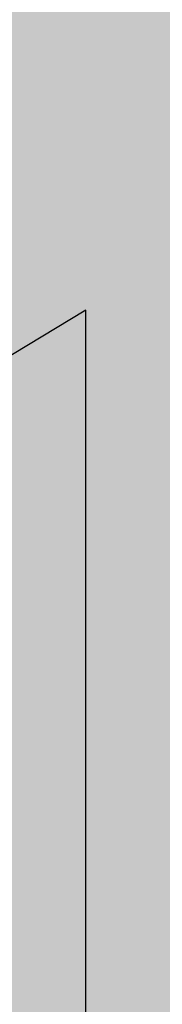
# Model space of a CAD drawing. Units: millimetres. Extents: x -22994 to 29398, y -19990 to 20176.
# Tile 79 of 135: x 225.272 to 225.543, y 85.199 to 87.071. Entities that reach past the tile are written whole.
import ezdxf
from ezdxf import colors
from ezdxf.entities.mleader import LeaderData, LeaderLine
from ezdxf.math import Vec2, Vec3

# ---------------------------------------------------------------- set-up
doc = ezdxf.new("R2010")
doc.units = ezdxf.units.MM
doc.header["$MEASUREMENT"] = 0
for name, color, linetype, lineweight in [('M-ANNO-TEXT', 7, 'Continuous', 25), ('M-DIMS', 2, 'Continuous', 18), ('M-EQPM', 7, 'Continuous', 25), ('M-EQPM-PATT', 7, 'Continuous', 18)]:
    doc.layers.add(name, color=color, linetype=linetype, lineweight=lineweight)
doc.styles.get("Standard").update_dxf_attribs({"font": 'arial.ttf'})
doc.dimstyles.get("Standard").update_dxf_attribs({"dimtxt": 0.18, "dimasz": 10000, "dimexe": 0.18, "dimexo": 0.0625, "dimgap": 0.09, "dimtad": 0, "dimtih": 1, "dimtoh": 1, "dimdec": 0, "dimzin": 0, "dimdsep": 46, "dimtxsty": 'Standard', "dimcen": 0.09, "dimadec": 0, "dimazin": 0, "dimtfac": 1, "dimtdec": 0, "dimtofl": 0, "dimtmove": 0, "dimatfit": 3, "dimfxl": 1, "dimtolj": 1, "dimtzin": 0, "dimlwd": 30, "dimarcsym": 0})

# ---------------------------------------------------------------- blocks, each defined once
blk = doc.blocks.new('*D2')
at = {"layer": 'Defpoints', "color": 0, "transparency": 16777216}
for p in [(6.6773, 10.2713), (290.852, 10.2713), (290.852, -5.0787)]:
    blk.add_point(p, dxfattribs=at)
at = {"layer": 'M-DIMS', "color": 0, "lineweight": -2, "transparency": 16777216}
for p, q in [((6.6773, 10.2088), (6.6773, -5.2587)), ((290.852, 10.2088), (290.852, -5.2587))]:
    blk.add_line(p, q, dxfattribs=at)
at = {"layer": 'M-DIMS', "color": 0, "lineweight": 30, "transparency": 16777216}
for p, q in [((-9993.3227, -5.0787), (-19993.3227, -5.0787)), ((10290.852, -5.0787), (20290.852, -5.0787))]:
    blk.add_line(p, q, dxfattribs=at)
at = {"layer": 'M-DIMS', "color": 0, "transparency": 16777216}
for points in [[(-9993.3227, 1661.5879), (-9993.3227, -1671.7454), (6.6773, -5.0787)], [(10290.852, 1661.5879), (10290.852, -1671.7454), (290.852, -5.0787)]]:
    blk.add_solid(points, dxfattribs=at)
at = {"layer": 'M-DIMS', "color": 0, "transparency": 16777216, "insert": (148.7647, -5.0787), "char_height": 0.18, "attachment_point": 5}
blk.add_mtext('\\A1;284.2', dxfattribs=at)
blk = doc.blocks.new('*D3')
at = {"layer": 'Defpoints', "color": 0, "transparency": 16777216}
for p in [(110.2647, 204.1654), (110.2647, 176.3662), (95.8327, 127.967)]:
    blk.add_point(p, dxfattribs=at)
at = {"layer": 'M-DIMS', "color": 0, "lineweight": -2, "transparency": 16777216}
for p, q in [((95.8327, 128.0295), (95.8327, 204.3454)), ((110.2647, 176.4287), (110.2647, 204.3454))]:
    blk.add_line(p, q, dxfattribs=at)
at = {"layer": 'M-DIMS', "color": 0, "lineweight": 30, "transparency": 16777216}
for p, q in [((-9904.1673, 204.1654), (-19904.1673, 204.1654)), ((10110.2647, 204.1654), (20110.2647, 204.1654))]:
    blk.add_line(p, q, dxfattribs=at)
at = {"layer": 'M-DIMS', "color": 0, "transparency": 16777216}
for points in [[(-9904.1673, 1870.8321), (-9904.1673, -1462.5013), (95.8327, 204.1654)], [(10110.2647, 1870.8321), (10110.2647, -1462.5013), (110.2647, 204.1654)]]:
    blk.add_solid(points, dxfattribs=at)
at = {"layer": 'M-DIMS', "color": 0, "transparency": 16777216, "insert": (103.0487, 204.1654), "char_height": 0.18, "attachment_point": 5}
blk.add_mtext('\\A1;14.432', dxfattribs=at)
blk = doc.blocks.new('*D4')
at = {"layer": 'Defpoints', "color": 0, "transparency": 16777216}
for p in [(116.2647, 204.1654), (110.2647, 176.3662), (116.2647, 176.3662)]:
    blk.add_point(p, dxfattribs=at)
at = {"layer": 'M-DIMS', "color": 0, "lineweight": -2, "transparency": 16777216}
for p, q in [((110.2647, 176.4287), (110.2647, 204.3454)), ((116.2647, 176.4287), (116.2647, 204.3454))]:
    blk.add_line(p, q, dxfattribs=at)
at = {"layer": 'M-DIMS', "color": 0, "lineweight": 30, "transparency": 16777216}
for p, q in [((-9889.7353, 204.1654), (-19889.7353, 204.1654)), ((10116.2647, 204.1654), (20116.2647, 204.1654))]:
    blk.add_line(p, q, dxfattribs=at)
at = {"layer": 'M-DIMS', "color": 0, "transparency": 16777216}
for points in [[(-9889.7353, 1870.8321), (-9889.7353, -1462.5013), (110.2647, 204.1654)], [(10116.2647, 1870.8321), (10116.2647, -1462.5013), (116.2647, 204.1654)]]:
    blk.add_solid(points, dxfattribs=at)
at = {"layer": 'M-DIMS', "color": 0, "transparency": 16777216, "insert": (113.2647, 204.1654), "char_height": 0.18, "attachment_point": 5}
blk.add_mtext('\\A1;6', dxfattribs=at)
blk = doc.blocks.new('*D5')
at = {"layer": 'Defpoints', "color": 0, "transparency": 16777216}
for p in [(181.2647, 204.1654), (116.2647, 176.3662), (181.2647, 176.3662)]:
    blk.add_point(p, dxfattribs=at)
at = {"layer": 'M-DIMS', "color": 0, "lineweight": -2, "transparency": 16777216}
for p, q in [((116.2647, 176.4287), (116.2647, 204.3454)), ((181.2647, 176.4287), (181.2647, 204.3454))]:
    blk.add_line(p, q, dxfattribs=at)
at = {"layer": 'M-DIMS', "color": 0, "lineweight": 30, "transparency": 16777216}
for p, q in [((-9883.7353, 204.1654), (-19883.7353, 204.1654)), ((10181.2647, 204.1654), (20181.2647, 204.1654))]:
    blk.add_line(p, q, dxfattribs=at)
at = {"layer": 'M-DIMS', "color": 0, "transparency": 16777216}
for points in [[(-9883.7353, 1870.8321), (-9883.7353, -1462.5013), (116.2647, 204.1654)], [(10181.2647, 1870.8321), (10181.2647, -1462.5013), (181.2647, 204.1654)]]:
    blk.add_solid(points, dxfattribs=at)
at = {"layer": 'M-DIMS', "color": 0, "transparency": 16777216, "insert": (148.7647, 204.1654), "char_height": 0.18, "attachment_point": 5}
blk.add_mtext('\\A1;65', dxfattribs=at)
blk = doc.blocks.new('*D6')
at = {"layer": 'Defpoints', "color": 0, "transparency": 16777216}
for p in [(187.2647, 204.1654), (181.2647, 176.3662), (187.2647, 176.3662)]:
    blk.add_point(p, dxfattribs=at)
at = {"layer": 'M-DIMS', "color": 0, "lineweight": -2, "transparency": 16777216}
for p, q in [((181.2647, 176.4287), (181.2647, 204.3454)), ((187.2647, 176.4287), (187.2647, 204.3454))]:
    blk.add_line(p, q, dxfattribs=at)
at = {"layer": 'M-DIMS', "color": 0, "lineweight": 30, "transparency": 16777216}
for p, q in [((-9818.7353, 204.1654), (-19818.7353, 204.1654)), ((10187.2647, 204.1654), (20187.2647, 204.1654))]:
    blk.add_line(p, q, dxfattribs=at)
at = {"layer": 'M-DIMS', "color": 0, "transparency": 16777216}
for points in [[(-9818.7353, 1870.8321), (-9818.7353, -1462.5013), (181.2647, 204.1654)], [(10187.2647, 1870.8321), (10187.2647, -1462.5013), (187.2647, 204.1654)]]:
    blk.add_solid(points, dxfattribs=at)
at = {"layer": 'M-DIMS', "color": 0, "transparency": 16777216, "insert": (184.2647, 204.1654), "char_height": 0.18, "attachment_point": 5}
blk.add_mtext('\\A1;6', dxfattribs=at)
blk = doc.blocks.new('*D7')
at = {"layer": 'Defpoints', "color": 0, "transparency": 16777216}
for p in [(201.6967, 204.1654), (187.2647, 176.3662), (201.6967, 127.967)]:
    blk.add_point(p, dxfattribs=at)
at = {"layer": 'M-DIMS', "color": 0, "lineweight": -2, "transparency": 16777216}
for p, q in [((187.2647, 176.4287), (187.2647, 204.3454)), ((201.6967, 128.0295), (201.6967, 204.3454))]:
    blk.add_line(p, q, dxfattribs=at)
at = {"layer": 'M-DIMS', "color": 0, "lineweight": 30, "transparency": 16777216}
for p, q in [((-9812.7353, 204.1654), (-19812.7353, 204.1654)), ((10201.6967, 204.1654), (20201.6967, 204.1654))]:
    blk.add_line(p, q, dxfattribs=at)
at = {"layer": 'M-DIMS', "color": 0, "transparency": 16777216}
for points in [[(-9812.7353, 1870.8321), (-9812.7353, -1462.5013), (187.2647, 204.1654)], [(10201.6967, 1870.8321), (10201.6967, -1462.5013), (201.6967, 204.1654)]]:
    blk.add_solid(points, dxfattribs=at)
at = {"layer": 'M-DIMS', "color": 0, "transparency": 16777216, "insert": (194.4807, 204.1654), "char_height": 0.18, "attachment_point": 5}
blk.add_mtext('\\A1;14.432', dxfattribs=at)
blk = doc.blocks.new('*D8')
at = {"layer": 'Defpoints', "color": 0, "transparency": 16777216}
for p in [(227.6485, 204.1654), (227.6485, 146.7296), (201.6967, 127.967)]:
    blk.add_point(p, dxfattribs=at)
at = {"layer": 'M-DIMS', "color": 0, "lineweight": -2, "transparency": 16777216}
for p, q in [((201.6967, 128.0295), (201.6967, 204.3454)), ((227.6485, 146.7921), (227.6485, 204.3454))]:
    blk.add_line(p, q, dxfattribs=at)
at = {"layer": 'M-DIMS', "color": 0, "lineweight": 30, "transparency": 16777216}
for p, q in [((-9798.3033, 204.1654), (-19798.3033, 204.1654)), ((10227.6485, 204.1654), (20227.6485, 204.1654))]:
    blk.add_line(p, q, dxfattribs=at)
at = {"layer": 'M-DIMS', "color": 0, "transparency": 16777216}
for points in [[(-9798.3033, 1870.8321), (-9798.3033, -1462.5013), (201.6967, 204.1654)], [(10227.6485, 1870.8321), (10227.6485, -1462.5013), (227.6485, 204.1654)]]:
    blk.add_solid(points, dxfattribs=at)
at = {"layer": 'M-DIMS', "color": 0, "transparency": 16777216, "insert": (214.6726, 204.1654), "char_height": 0.18, "attachment_point": 5}
blk.add_mtext('\\A1;25.95', dxfattribs=at)
blk = doc.blocks.new('*D9')
at = {"layer": 'Defpoints', "color": 0, "transparency": 16777216}
for p in [(187.2647, 176.3662), (306.202, 176.3662), (290.852, 10.2713)]:
    blk.add_point(p, dxfattribs=at)
at = {"layer": 'M-DIMS', "color": 0, "lineweight": 30, "transparency": 16777216}
for p, q in [((306.202, 10176.3662), (306.202, 20176.3662)), ((306.202, -9989.7287), (306.202, -19989.7287))]:
    blk.add_line(p, q, dxfattribs=at)
at = {"layer": 'M-DIMS', "color": 0, "lineweight": -2, "transparency": 16777216}
for p, q in [((187.3272, 176.3662), (306.382, 176.3662)), ((290.9145, 10.2713), (306.382, 10.2713))]:
    blk.add_line(p, q, dxfattribs=at)
at = {"layer": 'M-DIMS', "color": 0, "transparency": 16777216}
for points in [[(-1360.4646, 10176.3662), (1972.8687, 10176.3662), (306.202, 176.3662)], [(-1360.4646, -9989.7287), (1972.8687, -9989.7287), (306.202, 10.2713)]]:
    blk.add_solid(points, dxfattribs=at)
at = {"layer": 'M-DIMS', "color": 0, "transparency": 16777216, "insert": (306.202, 93.3187), "char_height": 0.18, "attachment_point": 5}
blk.add_mtext('\\A1;166.1', dxfattribs=at)
blk = doc.blocks.new('*D10')
at = {"layer": 'Defpoints', "color": 0, "transparency": 16777216}
for p in [(125.6498, 136.0713), (133.3459, 136.0713), (133.3459, -5.0787)]:
    blk.add_point(p, dxfattribs=at)
at = {"layer": 'M-DIMS', "color": 0, "lineweight": -2, "transparency": 16777216}
for p, q in [((125.6498, 136.0088), (125.6498, -5.2587)), ((133.3459, 136.0088), (133.3459, -5.2587))]:
    blk.add_line(p, q, dxfattribs=at)
at = {"layer": 'M-DIMS', "color": 0, "lineweight": 30, "transparency": 16777216}
for p, q in [((-9874.3502, -5.0787), (-19874.3502, -5.0787)), ((10133.3459, -5.0787), (20133.3459, -5.0787))]:
    blk.add_line(p, q, dxfattribs=at)
at = {"layer": 'M-DIMS', "color": 0, "transparency": 16777216}
for points in [[(-9874.3502, 1661.5879), (-9874.3502, -1671.7454), (125.6498, -5.0787)], [(10133.3459, 1661.5879), (10133.3459, -1671.7454), (133.3459, -5.0787)]]:
    blk.add_solid(points, dxfattribs=at)
at = {"layer": 'M-DIMS', "color": 0, "transparency": 16777216, "insert": (129.4978, -5.0787), "char_height": 0.18, "attachment_point": 5}
blk.add_mtext('\\A1;7.696', dxfattribs=at)
blk = doc.blocks.new('*D11')
at = {"layer": 'Defpoints', "color": 0, "transparency": 16777216}
for p in [(133.3459, 136.0713), (135.6498, 136.0713), (135.6498, -5.0787)]:
    blk.add_point(p, dxfattribs=at)
at = {"layer": 'M-DIMS', "color": 0, "lineweight": -2, "transparency": 16777216}
for p, q in [((133.3459, 136.0088), (133.3459, -5.2587)), ((135.6498, 136.0088), (135.6498, -5.2587))]:
    blk.add_line(p, q, dxfattribs=at)
at = {"layer": 'M-DIMS', "color": 0, "lineweight": 30, "transparency": 16777216}
for p, q in [((-9866.6541, -5.0787), (-19866.6541, -5.0787)), ((10135.6498, -5.0787), (20135.6498, -5.0787))]:
    blk.add_line(p, q, dxfattribs=at)
at = {"layer": 'M-DIMS', "color": 0, "transparency": 16777216}
for points in [[(-9866.6541, 1661.5879), (-9866.6541, -1671.7454), (133.3459, -5.0787)], [(10135.6498, 1661.5879), (10135.6498, -1671.7454), (135.6498, -5.0787)]]:
    blk.add_solid(points, dxfattribs=at)
at = {"layer": 'M-DIMS', "color": 0, "transparency": 16777216, "insert": (134.4978, -5.0787), "char_height": 0.18, "attachment_point": 5}
blk.add_mtext('\\A1;2.304', dxfattribs=at)
blk = doc.blocks.new('*D12')
at = {"layer": 'Defpoints', "color": 0, "transparency": 16777216}
for p in [(135.6498, 136.0713), (145.6498, 136.0713), (145.6498, -5.0787)]:
    blk.add_point(p, dxfattribs=at)
at = {"layer": 'M-DIMS', "color": 0, "lineweight": -2, "transparency": 16777216}
for p, q in [((135.6498, 136.0088), (135.6498, -5.2587)), ((145.6498, 136.0088), (145.6498, -5.2587))]:
    blk.add_line(p, q, dxfattribs=at)
at = {"layer": 'M-DIMS', "color": 0, "lineweight": 30, "transparency": 16777216}
for p, q in [((-9864.3502, -5.0787), (-19864.3502, -5.0787)), ((10145.6498, -5.0787), (20145.6498, -5.0787))]:
    blk.add_line(p, q, dxfattribs=at)
at = {"layer": 'M-DIMS', "color": 0, "transparency": 16777216}
for points in [[(-9864.3502, 1661.5879), (-9864.3502, -1671.7454), (135.6498, -5.0787)], [(10145.6498, 1661.5879), (10145.6498, -1671.7454), (145.6498, -5.0787)]]:
    blk.add_solid(points, dxfattribs=at)
at = {"layer": 'M-DIMS', "color": 0, "transparency": 16777216, "insert": (140.6498, -5.0787), "char_height": 0.18, "attachment_point": 5}
blk.add_mtext('\\A1;10', dxfattribs=at)
blk = doc.blocks.new('*D13')
at = {"layer": 'Defpoints', "color": 0, "transparency": 16777216}
for p in [(145.6498, 136.0713), (155.6498, 136.0713), (155.6498, -5.0787)]:
    blk.add_point(p, dxfattribs=at)
at = {"layer": 'M-DIMS', "color": 0, "lineweight": -2, "transparency": 16777216}
for p, q in [((145.6498, 136.0088), (145.6498, -5.2587)), ((155.6498, 136.0088), (155.6498, -5.2587))]:
    blk.add_line(p, q, dxfattribs=at)
at = {"layer": 'M-DIMS', "color": 0, "lineweight": 30, "transparency": 16777216}
for p, q in [((-9854.3502, -5.0787), (-19854.3502, -5.0787)), ((10155.6498, -5.0787), (20155.6498, -5.0787))]:
    blk.add_line(p, q, dxfattribs=at)
at = {"layer": 'M-DIMS', "color": 0, "transparency": 16777216}
for points in [[(-9854.3502, 1661.5879), (-9854.3502, -1671.7454), (145.6498, -5.0787)], [(10155.6498, 1661.5879), (10155.6498, -1671.7454), (155.6498, -5.0787)]]:
    blk.add_solid(points, dxfattribs=at)
at = {"layer": 'M-DIMS', "color": 0, "transparency": 16777216, "insert": (150.6498, -5.0787), "char_height": 0.18, "attachment_point": 5}
blk.add_mtext('\\A1;10', dxfattribs=at)
blk = doc.blocks.new('*D14')
at = {"layer": 'Defpoints', "color": 0, "transparency": 16777216}
for p in [(155.6498, 136.0713), (165.6498, 136.0713), (165.6498, -5.0787)]:
    blk.add_point(p, dxfattribs=at)
at = {"layer": 'M-DIMS', "color": 0, "lineweight": -2, "transparency": 16777216}
for p, q in [((155.6498, 136.0088), (155.6498, -5.2587)), ((165.6498, 136.0088), (165.6498, -5.2587))]:
    blk.add_line(p, q, dxfattribs=at)
at = {"layer": 'M-DIMS', "color": 0, "lineweight": 30, "transparency": 16777216}
for p, q in [((-9844.3502, -5.0787), (-19844.3502, -5.0787)), ((10165.6498, -5.0787), (20165.6498, -5.0787))]:
    blk.add_line(p, q, dxfattribs=at)
at = {"layer": 'M-DIMS', "color": 0, "transparency": 16777216}
for points in [[(-9844.3502, 1661.5879), (-9844.3502, -1671.7454), (155.6498, -5.0787)], [(10165.6498, 1661.5879), (10165.6498, -1671.7454), (165.6498, -5.0787)]]:
    blk.add_solid(points, dxfattribs=at)
at = {"layer": 'M-DIMS', "color": 0, "transparency": 16777216, "insert": (160.6498, -5.0787), "char_height": 0.18, "attachment_point": 5}
blk.add_mtext('\\A1;10', dxfattribs=at)
blk = doc.blocks.new('*D15')
at = {"layer": 'Defpoints', "color": 0, "transparency": 16777216}
for p in [(173.3459, 154.788), (173.3459, 136.0713), (306.202, 136.0713)]:
    blk.add_point(p, dxfattribs=at)
at = {"layer": 'M-DIMS', "color": 0, "lineweight": 30, "transparency": 16777216}
for p, q in [((306.202, 10154.788), (306.202, 20154.788)), ((306.202, -9863.9287), (306.202, -19863.9287))]:
    blk.add_line(p, q, dxfattribs=at)
at = {"layer": 'M-DIMS', "color": 0, "lineweight": -2, "transparency": 16777216}
for p, q in [((173.4084, 154.788), (306.382, 154.788)), ((173.4084, 136.0713), (306.382, 136.0713))]:
    blk.add_line(p, q, dxfattribs=at)
at = {"layer": 'M-DIMS', "color": 0, "transparency": 16777216}
for points in [[(-1360.4646, 10154.788), (1972.8687, 10154.788), (306.202, 154.788)], [(-1360.4646, -9863.9287), (1972.8687, -9863.9287), (306.202, 136.0713)]]:
    blk.add_solid(points, dxfattribs=at)
at = {"layer": 'M-DIMS', "color": 0, "transparency": 16777216, "insert": (306.202, 145.4297), "char_height": 0.18, "attachment_point": 5}
blk.add_mtext('\\A1;18.717', dxfattribs=at)
blk = doc.blocks.new('*D16')
at = {"layer": 'Defpoints', "color": 0, "transparency": 16777216}
for p in [(120.1702, 204.1654), (110.4658, 48.0349), (120.1702, 48.0349)]:
    blk.add_point(p, dxfattribs=at)
at = {"layer": 'M-DIMS', "color": 0, "lineweight": -2, "transparency": 16777216}
for p, q in [((110.4658, 48.0974), (110.4658, 204.3454)), ((120.1702, 48.0974), (120.1702, 204.3454))]:
    blk.add_line(p, q, dxfattribs=at)
at = {"layer": 'M-DIMS', "color": 0, "lineweight": 30, "transparency": 16777216}
for p, q in [((-9889.5342, 204.1654), (-19889.5342, 204.1654)), ((10120.1702, 204.1654), (20120.1702, 204.1654))]:
    blk.add_line(p, q, dxfattribs=at)
at = {"layer": 'M-DIMS', "color": 0, "transparency": 16777216}
for points in [[(-9889.5342, 1870.8321), (-9889.5342, -1462.5013), (110.4658, 204.1654)], [(10120.1702, 1870.8321), (10120.1702, -1462.5013), (120.1702, 204.1654)]]:
    blk.add_solid(points, dxfattribs=at)
at = {"layer": 'M-DIMS', "color": 0, "transparency": 16777216, "insert": (115.318, 204.1654), "char_height": 0.18, "attachment_point": 5}
blk.add_mtext('\\A1;9.704', dxfattribs=at)
blk = doc.blocks.new('*D17')
at = {"layer": 'Defpoints', "color": 0, "transparency": 16777216}
for p in [(126.1702, 204.1654), (120.1702, 48.0349), (126.1702, 48.0349)]:
    blk.add_point(p, dxfattribs=at)
at = {"layer": 'M-DIMS', "color": 0, "lineweight": -2, "transparency": 16777216}
for p, q in [((120.1702, 48.0974), (120.1702, 204.3454)), ((126.1702, 48.0974), (126.1702, 204.3454))]:
    blk.add_line(p, q, dxfattribs=at)
at = {"layer": 'M-DIMS', "color": 0, "lineweight": 30, "transparency": 16777216}
for p, q in [((-9879.8298, 204.1654), (-19879.8298, 204.1654)), ((10126.1702, 204.1654), (20126.1702, 204.1654))]:
    blk.add_line(p, q, dxfattribs=at)
at = {"layer": 'M-DIMS', "color": 0, "transparency": 16777216}
for points in [[(-9879.8298, 1870.8321), (-9879.8298, -1462.5013), (120.1702, 204.1654)], [(10126.1702, 1870.8321), (10126.1702, -1462.5013), (126.1702, 204.1654)]]:
    blk.add_solid(points, dxfattribs=at)
at = {"layer": 'M-DIMS', "color": 0, "transparency": 16777216, "insert": (123.1702, 204.1654), "char_height": 0.18, "attachment_point": 5}
blk.add_mtext('\\A1;6', dxfattribs=at)
blk = doc.blocks.new('*D18')
at = {"layer": 'Defpoints', "color": 0, "transparency": 16777216}
for p in [(132.1702, 204.1654), (126.1702, 48.0349), (132.1702, 48.0349)]:
    blk.add_point(p, dxfattribs=at)
at = {"layer": 'M-DIMS', "color": 0, "lineweight": -2, "transparency": 16777216}
for p, q in [((126.1702, 48.0974), (126.1702, 204.3454)), ((132.1702, 48.0974), (132.1702, 204.3454))]:
    blk.add_line(p, q, dxfattribs=at)
at = {"layer": 'M-DIMS', "color": 0, "lineweight": 30, "transparency": 16777216}
for p, q in [((-9873.8298, 204.1654), (-19873.8298, 204.1654)), ((10132.1702, 204.1654), (20132.1702, 204.1654))]:
    blk.add_line(p, q, dxfattribs=at)
at = {"layer": 'M-DIMS', "color": 0, "transparency": 16777216}
for points in [[(-9873.8298, 1870.8321), (-9873.8298, -1462.5013), (126.1702, 204.1654)], [(10132.1702, 1870.8321), (10132.1702, -1462.5013), (132.1702, 204.1654)]]:
    blk.add_solid(points, dxfattribs=at)
at = {"layer": 'M-DIMS', "color": 0, "transparency": 16777216, "insert": (129.1702, 204.1654), "char_height": 0.18, "attachment_point": 5}
blk.add_mtext('\\A1;6', dxfattribs=at)
blk = doc.blocks.new('*D19')
at = {"layer": 'Defpoints', "color": 0, "transparency": 16777216}
for p in [(138.1702, 204.1654), (132.1702, 48.0349), (138.1702, 48.0349)]:
    blk.add_point(p, dxfattribs=at)
at = {"layer": 'M-DIMS', "color": 0, "lineweight": -2, "transparency": 16777216}
for p, q in [((132.1702, 48.0974), (132.1702, 204.3454)), ((138.1702, 48.0974), (138.1702, 204.3454))]:
    blk.add_line(p, q, dxfattribs=at)
at = {"layer": 'M-DIMS', "color": 0, "lineweight": 30, "transparency": 16777216}
for p, q in [((-9867.8298, 204.1654), (-19867.8298, 204.1654)), ((10138.1702, 204.1654), (20138.1702, 204.1654))]:
    blk.add_line(p, q, dxfattribs=at)
at = {"layer": 'M-DIMS', "color": 0, "transparency": 16777216}
for points in [[(-9867.8298, 1870.8321), (-9867.8298, -1462.5013), (132.1702, 204.1654)], [(10138.1702, 1870.8321), (10138.1702, -1462.5013), (138.1702, 204.1654)]]:
    blk.add_solid(points, dxfattribs=at)
at = {"layer": 'M-DIMS', "color": 0, "transparency": 16777216, "insert": (135.1702, 204.1654), "char_height": 0.18, "attachment_point": 5}
blk.add_mtext('\\A1;6', dxfattribs=at)
blk = doc.blocks.new('*D20')
at = {"layer": 'Defpoints', "color": 0, "transparency": 16777216}
for p in [(144.1702, 204.1654), (138.1702, 48.0349), (144.1702, 48.0349)]:
    blk.add_point(p, dxfattribs=at)
at = {"layer": 'M-DIMS', "color": 0, "lineweight": -2, "transparency": 16777216}
for p, q in [((138.1702, 48.0974), (138.1702, 204.3454)), ((144.1702, 48.0974), (144.1702, 204.3454))]:
    blk.add_line(p, q, dxfattribs=at)
at = {"layer": 'M-DIMS', "color": 0, "lineweight": 30, "transparency": 16777216}
for p, q in [((-9861.8298, 204.1654), (-19861.8298, 204.1654)), ((10144.1702, 204.1654), (20144.1702, 204.1654))]:
    blk.add_line(p, q, dxfattribs=at)
at = {"layer": 'M-DIMS', "color": 0, "transparency": 16777216}
for points in [[(-9861.8298, 1870.8321), (-9861.8298, -1462.5013), (138.1702, 204.1654)], [(10144.1702, 1870.8321), (10144.1702, -1462.5013), (144.1702, 204.1654)]]:
    blk.add_solid(points, dxfattribs=at)
at = {"layer": 'M-DIMS', "color": 0, "transparency": 16777216, "insert": (141.1702, 204.1654), "char_height": 0.18, "attachment_point": 5}
blk.add_mtext('\\A1;6', dxfattribs=at)
blk = doc.blocks.new('*D21')
at = {"layer": 'Defpoints', "color": 0, "transparency": 16777216}
for p in [(149.1157, 204.1654), (144.1702, 48.0349), (149.1157, 48.0349)]:
    blk.add_point(p, dxfattribs=at)
at = {"layer": 'M-DIMS', "color": 0, "lineweight": -2, "transparency": 16777216}
for p, q in [((144.1702, 48.0974), (144.1702, 204.3454)), ((149.1157, 48.0974), (149.1157, 204.3454))]:
    blk.add_line(p, q, dxfattribs=at)
at = {"layer": 'M-DIMS', "color": 0, "lineweight": 30, "transparency": 16777216}
for p, q in [((-9855.8298, 204.1654), (-19855.8298, 204.1654)), ((10149.1157, 204.1654), (20149.1157, 204.1654))]:
    blk.add_line(p, q, dxfattribs=at)
at = {"layer": 'M-DIMS', "color": 0, "transparency": 16777216}
for points in [[(-9855.8298, 1870.8321), (-9855.8298, -1462.5013), (144.1702, 204.1654)], [(10149.1157, 1870.8321), (10149.1157, -1462.5013), (149.1157, 204.1654)]]:
    blk.add_solid(points, dxfattribs=at)
at = {"layer": 'M-DIMS', "color": 0, "transparency": 16777216, "insert": (146.6429, 204.1654), "char_height": 0.18, "attachment_point": 5}
blk.add_mtext('\\A1;4.945', dxfattribs=at)
blk = doc.blocks.new('*D22')
at = {"layer": 'Defpoints', "color": 0, "transparency": 16777216}
for p in [(149.1157, 30.9895), (155.1157, 30.9895), (155.1157, -5.0787)]:
    blk.add_point(p, dxfattribs=at)
at = {"layer": 'M-DIMS', "color": 0, "lineweight": -2, "transparency": 16777216}
for p, q in [((149.1157, 30.927), (149.1157, -5.2587)), ((155.1157, 30.927), (155.1157, -5.2587))]:
    blk.add_line(p, q, dxfattribs=at)
at = {"layer": 'M-DIMS', "color": 0, "lineweight": 30, "transparency": 16777216}
for p, q in [((-9850.8843, -5.0787), (-19850.8843, -5.0787)), ((10155.1157, -5.0787), (20155.1157, -5.0787))]:
    blk.add_line(p, q, dxfattribs=at)
at = {"layer": 'M-DIMS', "color": 0, "transparency": 16777216}
for points in [[(-9850.8843, 1661.5879), (-9850.8843, -1671.7454), (149.1157, -5.0787)], [(10155.1157, 1661.5879), (10155.1157, -1671.7454), (155.1157, -5.0787)]]:
    blk.add_solid(points, dxfattribs=at)
at = {"layer": 'M-DIMS', "color": 0, "transparency": 16777216, "insert": (152.1157, -5.0787), "char_height": 0.18, "attachment_point": 5}
blk.add_mtext('\\A1;6', dxfattribs=at)
blk = doc.blocks.new('*D23')
at = {"layer": 'Defpoints', "color": 0, "transparency": 16777216}
for p in [(155.1157, 30.9895), (161.1157, 30.9895), (161.1157, -5.0787)]:
    blk.add_point(p, dxfattribs=at)
at = {"layer": 'M-DIMS', "color": 0, "lineweight": -2, "transparency": 16777216}
for p, q in [((155.1157, 30.927), (155.1157, -5.2587)), ((161.1157, 30.927), (161.1157, -5.2587))]:
    blk.add_line(p, q, dxfattribs=at)
at = {"layer": 'M-DIMS', "color": 0, "lineweight": 30, "transparency": 16777216}
for p, q in [((-9844.8843, -5.0787), (-19844.8843, -5.0787)), ((10161.1157, -5.0787), (20161.1157, -5.0787))]:
    blk.add_line(p, q, dxfattribs=at)
at = {"layer": 'M-DIMS', "color": 0, "transparency": 16777216}
for points in [[(-9844.8843, 1661.5879), (-9844.8843, -1671.7454), (155.1157, -5.0787)], [(10161.1157, 1661.5879), (10161.1157, -1671.7454), (161.1157, -5.0787)]]:
    blk.add_solid(points, dxfattribs=at)
at = {"layer": 'M-DIMS', "color": 0, "transparency": 16777216, "insert": (158.1157, -5.0787), "char_height": 0.18, "attachment_point": 5}
blk.add_mtext('\\A1;6', dxfattribs=at)
blk = doc.blocks.new('*D24')
at = {"layer": 'Defpoints', "color": 0, "transparency": 16777216}
for p in [(161.1157, 30.9895), (166.4387, 30.9895), (166.4387, -5.0787)]:
    blk.add_point(p, dxfattribs=at)
at = {"layer": 'M-DIMS', "color": 0, "lineweight": -2, "transparency": 16777216}
for p, q in [((161.1157, 30.927), (161.1157, -5.2587)), ((166.4387, 30.927), (166.4387, -5.2587))]:
    blk.add_line(p, q, dxfattribs=at)
at = {"layer": 'M-DIMS', "color": 0, "lineweight": 30, "transparency": 16777216}
for p, q in [((-9838.8843, -5.0787), (-19838.8843, -5.0787)), ((10166.4387, -5.0787), (20166.4387, -5.0787))]:
    blk.add_line(p, q, dxfattribs=at)
at = {"layer": 'M-DIMS', "color": 0, "transparency": 16777216}
for points in [[(-9838.8843, 1661.5879), (-9838.8843, -1671.7454), (161.1157, -5.0787)], [(10166.4387, 1661.5879), (10166.4387, -1671.7454), (166.4387, -5.0787)]]:
    blk.add_solid(points, dxfattribs=at)
at = {"layer": 'M-DIMS', "color": 0, "transparency": 16777216, "insert": (163.7772, -5.0787), "char_height": 0.18, "attachment_point": 5}
blk.add_mtext('\\A1;5.323', dxfattribs=at)
blk = doc.blocks.new('*D25')
at = {"layer": 'Defpoints', "color": 0, "transparency": 16777216}
for p in [(166.4387, 30.9895), (172.4387, 30.9895), (172.4387, -5.0787)]:
    blk.add_point(p, dxfattribs=at)
at = {"layer": 'M-DIMS', "color": 0, "lineweight": -2, "transparency": 16777216}
for p, q in [((166.4387, 30.927), (166.4387, -5.2587)), ((172.4387, 30.927), (172.4387, -5.2587))]:
    blk.add_line(p, q, dxfattribs=at)
at = {"layer": 'M-DIMS', "color": 0, "lineweight": 30, "transparency": 16777216}
for p, q in [((-9833.5613, -5.0787), (-19833.5613, -5.0787)), ((10172.4387, -5.0787), (20172.4387, -5.0787))]:
    blk.add_line(p, q, dxfattribs=at)
at = {"layer": 'M-DIMS', "color": 0, "transparency": 16777216}
for points in [[(-9833.5613, 1661.5879), (-9833.5613, -1671.7454), (166.4387, -5.0787)], [(10172.4387, 1661.5879), (10172.4387, -1671.7454), (172.4387, -5.0787)]]:
    blk.add_solid(points, dxfattribs=at)
at = {"layer": 'M-DIMS', "color": 0, "transparency": 16777216, "insert": (169.4387, -5.0787), "char_height": 0.18, "attachment_point": 5}
blk.add_mtext('\\A1;6', dxfattribs=at)
blk = doc.blocks.new('*D26')
at = {"layer": 'Defpoints', "color": 0, "transparency": 16777216}
for p in [(172.4387, 30.9895), (178.4387, 30.9895), (178.4387, -5.0787)]:
    blk.add_point(p, dxfattribs=at)
at = {"layer": 'M-DIMS', "color": 0, "lineweight": -2, "transparency": 16777216}
for p, q in [((172.4387, 30.927), (172.4387, -5.2587)), ((178.4387, 30.927), (178.4387, -5.2587))]:
    blk.add_line(p, q, dxfattribs=at)
at = {"layer": 'M-DIMS', "color": 0, "lineweight": 30, "transparency": 16777216}
for p, q in [((-9827.5613, -5.0787), (-19827.5613, -5.0787)), ((10178.4387, -5.0787), (20178.4387, -5.0787))]:
    blk.add_line(p, q, dxfattribs=at)
at = {"layer": 'M-DIMS', "color": 0, "transparency": 16777216}
for points in [[(-9827.5613, 1661.5879), (-9827.5613, -1671.7454), (172.4387, -5.0787)], [(10178.4387, 1661.5879), (10178.4387, -1671.7454), (178.4387, -5.0787)]]:
    blk.add_solid(points, dxfattribs=at)
at = {"layer": 'M-DIMS', "color": 0, "transparency": 16777216, "insert": (175.4387, -5.0787), "char_height": 0.18, "attachment_point": 5}
blk.add_mtext('\\A1;6', dxfattribs=at)
blk = doc.blocks.new('*D27')
at = {"layer": 'Defpoints', "color": 0, "transparency": 16777216}
for p in [(178.4387, 30.9895), (188.1175, 30.9895), (188.1175, -5.0787)]:
    blk.add_point(p, dxfattribs=at)
at = {"layer": 'M-DIMS', "color": 0, "lineweight": -2, "transparency": 16777216}
for p, q in [((178.4387, 30.927), (178.4387, -5.2587)), ((188.1175, 30.927), (188.1175, -5.2587))]:
    blk.add_line(p, q, dxfattribs=at)
at = {"layer": 'M-DIMS', "color": 0, "lineweight": 30, "transparency": 16777216}
for p, q in [((-9821.5613, -5.0787), (-19821.5613, -5.0787)), ((10188.1175, -5.0787), (20188.1175, -5.0787))]:
    blk.add_line(p, q, dxfattribs=at)
at = {"layer": 'M-DIMS', "color": 0, "transparency": 16777216}
for points in [[(-9821.5613, 1661.5879), (-9821.5613, -1671.7454), (178.4387, -5.0787)], [(10188.1175, 1661.5879), (10188.1175, -1671.7454), (188.1175, -5.0787)]]:
    blk.add_solid(points, dxfattribs=at)
at = {"layer": 'M-DIMS', "color": 0, "transparency": 16777216, "insert": (183.2781, -5.0787), "char_height": 0.18, "attachment_point": 5}
blk.add_mtext('\\A1;9.679', dxfattribs=at)
blk = doc.blocks.new('*D28')
at = {"layer": 'Defpoints', "color": 0, "transparency": 16777216}
for p in [(188.1175, 48.0349), (306.202, 48.0349), (188.1175, 30.9895)]:
    blk.add_point(p, dxfattribs=at)
at = {"layer": 'M-DIMS', "color": 0, "lineweight": 30, "transparency": 16777216}
for p, q in [((306.202, 10048.0349), (306.202, 20048.0349)), ((306.202, -9969.0105), (306.202, -19969.0105))]:
    blk.add_line(p, q, dxfattribs=at)
at = {"layer": 'M-DIMS', "color": 0, "lineweight": -2, "transparency": 16777216}
for p, q in [((188.18, 48.0349), (306.382, 48.0349)), ((188.18, 30.9895), (306.382, 30.9895))]:
    blk.add_line(p, q, dxfattribs=at)
at = {"layer": 'M-DIMS', "color": 0, "transparency": 16777216}
for points in [[(-1360.4646, 10048.0349), (1972.8687, 10048.0349), (306.202, 48.0349)], [(-1360.4646, -9969.0105), (1972.8687, -9969.0105), (306.202, 30.9895)]]:
    blk.add_solid(points, dxfattribs=at)
at = {"layer": 'M-DIMS', "color": 0, "transparency": 16777216, "insert": (306.202, 39.5122), "char_height": 0.18, "attachment_point": 5}
blk.add_mtext('\\A1;17.045', dxfattribs=at)
blk = doc.blocks.new('*D29')
at = {"layer": 'Defpoints', "color": 0, "transparency": 16777216}
for p in [(36.8006, 80.045), (64.0296, 80.045)]:
    blk.add_point(p, dxfattribs=at)
at = {"layer": 'M-DIMS', "color": 0, "lineweight": -2, "transparency": 16777216}
for p, q in [((50.4151, 79.955), (50.4151, 80.135)), ((50.3251, 80.045), (50.5051, 80.045))]:
    blk.add_line(p, q, dxfattribs=at)
at = {"layer": 'M-DIMS', "color": 0, "lineweight": 30, "transparency": 16777216}
blk.add_line((20064.0296, 80.0303), (10064.0296, 80.0377), dxfattribs=at)
at = {"layer": 'M-DIMS', "color": 0, "transparency": 16777216}
blk.add_solid([(10064.0309, 1746.7043), (10064.0284, -1586.629), (64.0296, 80.045)], dxfattribs=at)
at = {"layer": 'M-DIMS', "color": 0, "transparency": 16777216, "insert": (20064.5213, 80.0303), "char_height": 0.18, "attachment_point": 5}
blk.add_mtext('\\A1;∅27.23', dxfattribs=at)
blk = doc.blocks.new('*D30')
at = {"layer": 'Defpoints', "color": 0, "transparency": 16777216}
for p in [(216.3148, 146.7291), (238.9821, 146.73)]:
    blk.add_point(p, dxfattribs=at)
at = {"layer": 'M-DIMS', "color": 0, "lineweight": 30, "transparency": 16777216}
blk.add_line((20238.9821, 147.4959), (10238.9821, 147.1129), dxfattribs=at)
at = {"layer": 'M-DIMS', "color": 0, "lineweight": -2, "transparency": 16777216}
for p, q in [((227.6485, 146.6396), (227.6485, 146.8196)), ((227.5585, 146.7296), (227.7385, 146.7296))]:
    blk.add_line(p, q, dxfattribs=at)
at = {"layer": 'M-DIMS', "color": 0, "transparency": 16777216}
blk.add_solid([(10238.9183, 1813.7796), (10239.0459, -1519.5537), (238.9821, 146.73)], dxfattribs=at)
at = {"layer": 'M-DIMS', "color": 0, "transparency": 16777216, "insert": (20239.5436, 147.4959), "char_height": 0.18, "attachment_point": 5}
blk.add_mtext('\\A1;∅22.667', dxfattribs=at)
blk = doc.blocks.new('*D31')
at = {"layer": 'Defpoints', "color": 0, "transparency": 16777216}
for p in [(223.1641, 146.7291), (232.1328, 146.73)]:
    blk.add_point(p, dxfattribs=at)
at = {"layer": 'M-DIMS', "color": 0, "lineweight": 30, "transparency": 16777216}
blk.add_line((20232.1327, 148.6656), (10232.1328, 147.6978), dxfattribs=at)
at = {"layer": 'M-DIMS', "color": 0, "lineweight": -2, "transparency": 16777216}
for p, q in [((227.6485, 146.6396), (227.6485, 146.8196)), ((227.5585, 146.7296), (227.7385, 146.7296))]:
    blk.add_line(p, q, dxfattribs=at)
at = {"layer": 'M-DIMS', "color": 0, "transparency": 16777216}
blk.add_solid([(10231.9715, 1814.3645), (10232.2941, -1518.9688), (232.1328, 146.73)], dxfattribs=at)
at = {"layer": 'M-DIMS', "color": 0, "transparency": 16777216, "insert": (20232.6245, 148.6656), "char_height": 0.18, "attachment_point": 5}
blk.add_mtext('\\A1;∅8.969', dxfattribs=at)
blk = doc.blocks.new('*D36')
at = {"layer": 'Defpoints', "color": 0, "transparency": 16777216}
for p in [(46.39, 31.3035), (46.3875, 26.5934)]:
    blk.add_point(p, dxfattribs=at)
at = {"layer": 'M-DIMS', "color": 0, "lineweight": 30, "transparency": 16777216}
for p, q in [((57.1499, 20031.3006), (51.77, 10031.302)), ((10057.1499, 20031.3006), (57.1499, 20031.3006))]:
    blk.add_line(p, q, dxfattribs=at)
at = {"layer": 'M-DIMS', "color": 0, "lineweight": -2, "transparency": 16777216}
for p, q in [((46.3887, 28.8585), (46.3887, 29.0385)), ((46.2987, 28.9485), (46.4787, 28.9485))]:
    blk.add_line(p, q, dxfattribs=at)
at = {"layer": 'M-DIMS', "color": 0, "transparency": 16777216}
blk.add_solid([(-1614.8965, 10032.1987), (1718.4364, 10030.4054), (46.39, 31.3035)], dxfattribs=at)
at = {"layer": 'M-DIMS', "color": 0, "transparency": 16777216, "insert": (10057.5542, 20031.3006), "char_height": 0.18, "attachment_point": 5}
blk.add_mtext('\\A1;∅4.71', dxfattribs=at)
blk = doc.blocks.new('*D37')
at = {"layer": 'Defpoints', "color": 0, "transparency": 16777216}
for p in [(54.8343, 118.6145), (59.4936, 118.614)]:
    blk.add_point(p, dxfattribs=at)
at = {"layer": 'M-DIMS', "color": 0, "lineweight": -2, "transparency": 16777216}
for p, q in [((57.1639, 118.5243), (57.1639, 118.7043)), ((57.0739, 118.6143), (57.2539, 118.6143))]:
    blk.add_line(p, q, dxfattribs=at)
at = {"layer": 'M-DIMS', "color": 0, "lineweight": 30, "transparency": 16777216}
blk.add_line((20059.4934, 116.2531), (10059.4935, 117.4336), dxfattribs=at)
at = {"layer": 'M-DIMS', "color": 0, "transparency": 16777216}
blk.add_solid([(10059.6902, 1784.1002), (10059.2968, -1549.2331), (59.4936, 118.614)], dxfattribs=at)
at = {"layer": 'M-DIMS', "color": 0, "transparency": 16777216, "insert": (20059.9852, 116.2531), "char_height": 0.18, "attachment_point": 5}
blk.add_mtext('\\A1;∅4.659', dxfattribs=at)

msp = doc.modelspace()

# ---------------------------------------------------------------- hatches: boundary and pattern name
at = {"layer": 'M-EQPM-PATT'}
h = msp.add_hatch(color=256, dxfattribs=at)
h.set_gradient(color1=(205, 32, 39), color2=(205, 32, 39), tint=1)
h.paths.add_polyline_path([(116.2647, 150.3662), (116.2647, 170.3662), (116.2647, 176.3662), (110.2647, 176.3662), (110.2647, 152.0276), (95.8327, 127.967), (95.8327, 16.6063), (201.6967, 16.6063), (201.6967, 127.967), (187.2647, 152.0276), (187.2647, 176.3662), (181.2647, 176.3662), (181.2647, 170.3662), (181.2647, 150.3662), (195.6967, 126.3055), (195.6967, 22.6063), (101.8327, 22.6063), (101.8327, 126.3055)])
h.paths.add_polyline_path([(185.2208, 88.6347), (101.8327, 88.6347), (101.8327, 87.6347), (182.8066, 87.6347), (178.7313, 83.5594), (195.6967, 83.5594), (195.6967, 84.5594), (181.1455, 84.5594)], flags=17)
h.paths.add_polyline_path([(95.8327, 88.6347), (60.9779, 88.6347, -0.022855), (61.7178, 87.6347), (95.8327, 87.6347)])
h.paths.add_polyline_path([(215.6212, 86.5189), (215.6212, 80.5999), (220.5095, 83.5594)])
h.paths.add_polyline_path([(215.6212, 84.5594), (201.6967, 84.5594), (201.6967, 83.5594), (215.6212, 83.5594)])
h.paths.add_polyline_path([(225.3978, 86.5189), (220.5095, 83.5594), (225.3978, 80.5999)])
h.paths.add_polyline_path([(231.6256, 84.5594), (225.3978, 84.5594), (225.3978, 83.5594), (231.6256, 83.5594)])

# ---------------------------------------------------------------- linework, layer by layer
at = {"layer": 'M-EQPM'}
msp.add_lwpolyline([(225.3978, 86.5189), (215.6212, 80.5999), (215.6212, 86.5189), (225.3978, 80.5999)], close=True, dxfattribs=at)

# ---------------------------------------------------------------- dimensions: what is measured, and where the dimension line sits
at = {"layer": 'M-DIMS'}
for base, p1, p2, override, picture, middle in [((306.202, 176.3662), (290.852, 10.2713), (187.2647, 176.3662), {"dimdec": 1, "dimlfac": 1, "dimrnd": 0, "dimzin": 0, "dimdsep": 46, "dimlunit": 2}, '*D9', (306.202, 93.3187)), ((306.202, 136.0713), (173.3459, 154.788), (173.3459, 136.0713), {"dimdec": 3, "dimlfac": 1, "dimrnd": 0, "dimzin": 0, "dimdsep": 46, "dimlunit": 2}, '*D15', (306.202, 145.4297)), ((306.202, 48.0349), (188.1175, 30.9895), (188.1175, 48.0349), {"dimdec": 3, "dimlfac": 1, "dimrnd": 0, "dimzin": 0, "dimdsep": 46, "dimlunit": 2}, '*D28', (306.202, 39.5122))]:
    dim = msp.add_linear_dim(base=base, p1=p1, p2=p2, angle=90, dimstyle='Standard', override=override, dxfattribs=at)
    dim.commit()
    dim.dimension.update_dxf_attribs({"geometry": picture, "text_midpoint": middle})
for p1, p2, override, picture, middle in [((46.3875, 26.5934), (46.39, 31.3035), {"dimdec": 2, "dimlfac": 1, "dimrnd": 0, "dimzin": 0, "dimdsep": 46, "dimlunit": 2}, '*D36', (10057.5542, 20031.3006)), ((223.1641, 146.7291), (232.1328, 146.73), {"dimdec": 3, "dimlfac": 1, "dimrnd": 0, "dimzin": 0, "dimdsep": 46, "dimlunit": 2}, '*D31', (20232.1327, 148.6656)), ((216.3148, 146.7291), (238.9821, 146.73), {"dimdec": 3, "dimlfac": 1, "dimrnd": 0, "dimzin": 0, "dimdsep": 46, "dimlunit": 2}, '*D30', (20238.9821, 147.4959))]:
    dim = msp.add_diameter_dim_2p(p1=p1, p2=p2, dimstyle='Standard', override=override, dxfattribs=at)
    dim.commit()
    dim.dimension.update_dxf_attribs({"geometry": picture, "text_midpoint": middle, "dimtype": 163})
for base, p1, p2, override, picture, middle in [((110.2647, 204.1654), (95.8327, 127.967), (110.2647, 176.3662), {"dimdec": 3, "dimlfac": 1, "dimrnd": 0, "dimzin": 0, "dimdsep": 46, "dimlunit": 2}, '*D3', (103.0487, 204.1654)), ((116.2647, 204.1654), (110.2647, 176.3662), (116.2647, 176.3662), {"dimdec": 0, "dimlfac": 1, "dimrnd": 0, "dimzin": 0, "dimdsep": 46, "dimlunit": 2}, '*D4', (113.2647, 204.1654)), ((120.1702, 204.1654), (110.4658, 48.0349), (120.1702, 48.0349), {"dimdec": 3, "dimlfac": 1, "dimrnd": 0, "dimzin": 0, "dimdsep": 46, "dimlunit": 2}, '*D16', (115.318, 204.1654)), ((181.2647, 204.1654), (116.2647, 176.3662), (181.2647, 176.3662), {"dimdec": 0, "dimlfac": 1, "dimrnd": 0, "dimzin": 0, "dimdsep": 46, "dimlunit": 2}, '*D5', (148.7647, 204.1654)), ((126.1702, 204.1654), (120.1702, 48.0349), (126.1702, 48.0349), {"dimdec": 0, "dimlfac": 1, "dimrnd": 0, "dimzin": 0, "dimdsep": 46, "dimlunit": 2}, '*D17', (123.1702, 204.1654)), ((132.1702, 204.1654), (126.1702, 48.0349), (132.1702, 48.0349), {"dimdec": 0, "dimlfac": 1, "dimrnd": 0, "dimzin": 0, "dimdsep": 46, "dimlunit": 2}, '*D18', (129.1702, 204.1654)), ((138.1702, 204.1654), (132.1702, 48.0349), (138.1702, 48.0349), {"dimdec": 0, "dimlfac": 1, "dimrnd": 0, "dimzin": 0, "dimdsep": 46, "dimlunit": 2}, '*D19', (135.1702, 204.1654)), ((144.1702, 204.1654), (138.1702, 48.0349), (144.1702, 48.0349), {"dimdec": 0, "dimlfac": 1, "dimrnd": 0, "dimzin": 0, "dimdsep": 46, "dimlunit": 2}, '*D20', (141.1702, 204.1654)), ((149.11567, 204.16539), (144.17023, 48.03494), (149.11567, 48.03494), {"dimdec": 3, "dimlfac": 1, "dimrnd": 0, "dimzin": 0, "dimdsep": 46, "dimlunit": 2}, '*D21', (146.64295, 204.16539)), ((187.2647, 204.1654), (181.2647, 176.3662), (187.2647, 176.3662), {"dimdec": 0, "dimlfac": 1, "dimrnd": 0, "dimzin": 0, "dimdsep": 46, "dimlunit": 2}, '*D6', (184.2647, 204.1654)), ((201.6967, 204.1654), (187.2647, 176.3662), (201.6967, 127.967), {"dimdec": 3, "dimlfac": 1, "dimrnd": 0, "dimzin": 0, "dimdsep": 46, "dimlunit": 2}, '*D7', (194.4807, 204.1654)), ((227.6485, 204.1654), (201.6967, 127.967), (227.6485, 146.7296), {"dimdec": 2, "dimlfac": 1, "dimrnd": 0, "dimzin": 0, "dimdsep": 46, "dimlunit": 2}, '*D8', (214.6726, 204.1654)), ((290.852, -5.0787), (6.6773, 10.2713), (290.852, 10.2713), {"dimdec": 1, "dimlfac": 1, "dimrnd": 0, "dimzin": 0, "dimdsep": 46, "dimlunit": 2}, '*D2', (148.7647, -5.0787)), ((133.3459, -5.0787), (125.6498, 136.0713), (133.3459, 136.0713), {"dimdec": 3, "dimlfac": 1, "dimrnd": 0, "dimzin": 0, "dimdsep": 46, "dimlunit": 2}, '*D10', (129.4978, -5.0787)), ((135.6498, -5.0787), (133.3459, 136.0713), (135.6498, 136.0713), {"dimdec": 3, "dimlfac": 1, "dimrnd": 0, "dimzin": 0, "dimdsep": 46, "dimlunit": 2}, '*D11', (134.4978, -5.0787)), ((145.6498, -5.0787), (135.6498, 136.0713), (145.6498, 136.0713), {"dimdec": 0, "dimlfac": 1, "dimrnd": 0, "dimzin": 0, "dimdsep": 46, "dimlunit": 2}, '*D12', (140.6498, -5.0787)), ((155.6498, -5.0787), (145.6498, 136.0713), (155.6498, 136.0713), {"dimdec": 0, "dimlfac": 1, "dimrnd": 0, "dimzin": 0, "dimdsep": 46, "dimlunit": 2}, '*D13', (150.6498, -5.0787)), ((155.1157, -5.0787), (149.1157, 30.9895), (155.1157, 30.9895), {"dimdec": 0, "dimlfac": 1, "dimrnd": 0, "dimzin": 0, "dimdsep": 46, "dimlunit": 2}, '*D22', (152.1157, -5.0787)), ((161.1157, -5.0787), (155.1157, 30.9895), (161.1157, 30.9895), {"dimdec": 0, "dimlfac": 1, "dimrnd": 0, "dimzin": 0, "dimdsep": 46, "dimlunit": 2}, '*D23', (158.1157, -5.0787)), ((165.6498, -5.0787), (155.6498, 136.0713), (165.6498, 136.0713), {"dimdec": 0, "dimlfac": 1, "dimrnd": 0, "dimzin": 0, "dimdsep": 46, "dimlunit": 2}, '*D14', (160.6498, -5.0787)), ((166.4387, -5.0787), (161.1157, 30.9895), (166.4387, 30.9895), {"dimdec": 3, "dimlfac": 1, "dimrnd": 0, "dimzin": 0, "dimdsep": 46, "dimlunit": 2}, '*D24', (163.7772, -5.0787)), ((172.4387, -5.0787), (166.4387, 30.9895), (172.4387, 30.9895), {"dimdec": 0, "dimlfac": 1, "dimrnd": 0, "dimzin": 0, "dimdsep": 46, "dimlunit": 2}, '*D25', (169.4387, -5.0787)), ((178.4387, -5.0787), (172.4387, 30.9895), (178.4387, 30.9895), {"dimdec": 0, "dimlfac": 1, "dimrnd": 0, "dimzin": 0, "dimdsep": 46, "dimlunit": 2}, '*D26', (175.4387, -5.0787)), ((188.1175, -5.0787), (178.4387, 30.9895), (188.1175, 30.9895), {"dimdec": 3, "dimlfac": 1, "dimrnd": 0, "dimzin": 0, "dimdsep": 46, "dimlunit": 2}, '*D27', (183.2781, -5.0787))]:
    dim = msp.add_linear_dim(base=base, p1=p1, p2=p2, dimstyle='Standard', override=override, dxfattribs=at)
    dim.commit()
    dim.dimension.update_dxf_attribs({"geometry": picture, "text_midpoint": middle})
for p1, p2, override, picture, middle in [((54.8343, 118.6145), (59.4936, 118.614), {"dimdec": 3, "dimlfac": 1, "dimrnd": 0, "dimzin": 0, "dimdsep": 46, "dimlunit": 2}, '*D37', (20059.4934, 116.2531)), ((36.8006, 80.045), (64.0296, 80.045), {"dimdec": 2, "dimlfac": 1, "dimrnd": 0, "dimzin": 0, "dimdsep": 46, "dimlunit": 2}, '*D29', (20064.0296, 80.0303))]:
    dim = msp.add_diameter_dim_2p(p1=p1, p2=p2, dimstyle='Standard', override=override, dxfattribs=at)
    dim.commit()
    dim.dimension.update_dxf_attribs({"geometry": picture, "text_midpoint": middle})

# ---------------------------------------------------------------- leaders
at = {"layer": 'M-ANNO-TEXT'}
ml = msp.add_multileader_mtext('Standard', dxfattribs=at)
ml.set_content('combustion chamber', color=256)
ml.set_leader_properties()
ml.build(insert=Vec2(0, 0))
ml.multileader.update_dxf_attribs({"dogleg_length": 0.36, "arrow_head_size": 200})
ctx = ml.context
ctx.base_point, ctx.char_height, ctx.arrow_head_size, ctx.landing_gap_size, ctx.plane_origin = Vec3(215.7321, 57.9149), 3, 200, 0.09, Vec3(189.1175, 57.9149)
notes = []
notes.append((ctx, [(0, (1, 1, 0), (215.3721, 57.9149), (1, 0), 0.36, [(0, [(189.1175, 57.9149)], 0, [])])]))
ctx.mtext.insert, ctx.mtext.flow_direction = Vec3(215.8221, 59.4394), 5
for ctx, leaders in notes:
    for number, flags, end, landing, length, lines in leaders:
        leader = LeaderData()
        leader.index, (leader.has_last_leader_line, leader.has_dogleg_vector, leader.attachment_direction) = number, flags
        leader.last_leader_point, leader.dogleg_vector, leader.dogleg_length = Vec3(end), Vec3(landing), length
        for number, points, colour, breaks in lines:
            line = LeaderLine()
            line.index, line.vertices, line.color, line.breaks = number, Vec3.list(points), colors.encode_raw_color(colour), breaks
            leader.lines.append(line)
        ctx.leaders.append(leader)

doc.saveas('drawing.dxf')
